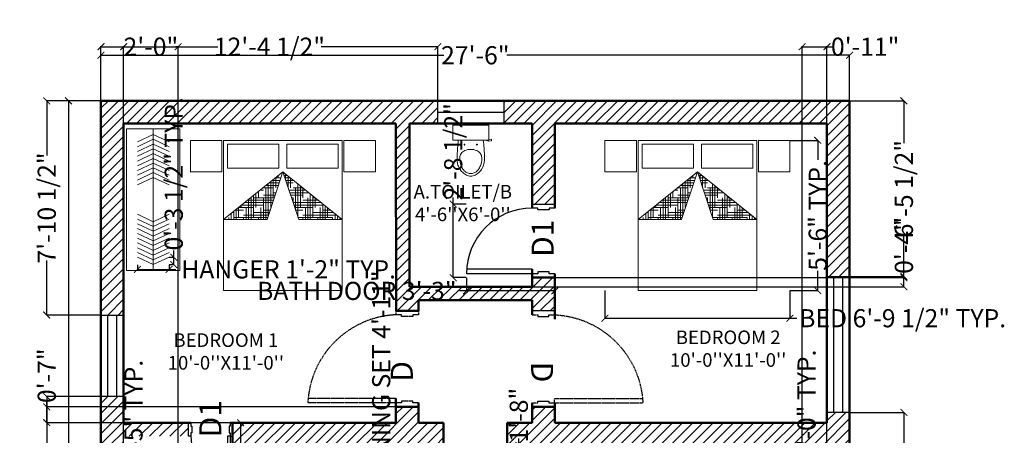
# Model space of a CAD drawing. Units: inches. Extents: x 1945 to 2401, y 1770 to 2289.
# Tile 5 of 5: x 1967 to 2401, y 2105 to 2289. Entities that reach past the tile are written whole.
import ezdxf

# ---------------------------------------------------------------- set-up
doc = ezdxf.new("R2010")
doc.units = ezdxf.units.IN
doc.linetypes.add('HIDDEN', pattern=[9.525, 6.35, -3.175])
for name, color, linetype, lineweight in [('A-ANNO-DIMS', 2, 'Continuous', 18), ('A-ANNO-TEXT', 7, 'Continuous', 18), ('A-AREA-IDEN', 7, 'Continuous', 25), ('A-DOOR-HIDN', 150, 'HIDDEN', 25), ('A-FLOR-FIXT', 9, 'Continuous', 18), ('A-WALL-PATT', 8, 'Continuous', 13), ('B-FURNITURE', 22, 'Continuous', 18), ('Doors', 150, 'Continuous', 25), ('shelves', 52, 'Continuous', 18), ('Walls', 7, 'Continuous', 50), ('Windows', 32, 'Continuous', 25)]:
    doc.layers.add(name, color=color, linetype=linetype, lineweight=lineweight)
doc.styles.get("Standard").update_dxf_attribs({"font": 'arial.ttf'})
doc.dimstyles.get("Standard").update_dxf_attribs({"dimtxt": 8, "dimasz": 3, "dimexe": 0.18, "dimexo": 0.0625, "dimgap": 0.09, "dimtad": 0, "dimdec": 1, "dimzin": 0, "dimdsep": 46, "dimlunit": 4, "dimtxsty": 'Standard', "dimblk": 'ARCHTICK', "dimcen": 0.09, "dimadec": 0, "dimazin": 0, "dimtfac": 1, "dimtdec": 1, "dimtofl": 0, "dimtmove": 0, "dimatfit": 3, "dimfxl": 1, "dimtolj": 1, "dimtzin": 0, "dimarcsym": 0})

# ---------------------------------------------------------------- blocks, each defined once
blk = doc.blocks.new('toilet-1')
at = {"color": 0, "linetype": 'ByBlock'}
for p, q in [((-0.23, -0.02), (-0.23, -0.212)), ((0.23, -0.02), (-0.23, -0.02)), ((0.23, -0.02), (0.23, -0.212)), ((-0.23, -0.212), (0.23, -0.212)), ((0.192, -0.214), (0.221, -0.225)), ((0.221, -0.225), (0.266, -0.219)), ((0.263, -0.2), (0.23, -0.204)), ((0.266, -0.219), (0.263, -0.2)), ((-0.089, -0.268), (-0.07, -0.268)), ((-0.079, -0.259), (-0.079, -0.278)), ((0.089, -0.268), (0.07, -0.268)), ((0.079, -0.259), (0.079, -0.278)), ((0, -0.638), (0, -0.638))]:
    blk.add_line(p, q, dxfattribs=at)
for centre, radius, start, end in [((3.527, -0.624), 3.709, 173.6925, 175.1593), ((-3.527, -0.624), 3.709, 4.8413, 6.3171), ((1.737, -0.452), 1.911, 175.7698, 180.3758), ((-0.031, -0.446), 0.111, 113.8997, 145.1485), ((0, -0.517), 0.188, 66.0939, 113.9061), ((0.031, -0.446), 0.111, 34.8515, 66.1003), ((-1.737, -0.452), 1.911, 359.6242, 4.2302), ((0.035, -0.463), 0.209, 180.3747, 194.3375), ((0.098, -0.45), 0.239, 175.8862, 195.5931), ((-0.041, -0.44), 0.0996, 145.1497, 175.881), ((0.041, -0.44), 0.0996, 4.119, 34.8503), ((-0.098, -0.45), 0.239, 344.4069, 4.1138), ((-0.035, -0.463), 0.209, 345.6614, 359.6243), ((0.055, -0.458), 0.23, 194.3353, 209.622), ((0.065, -0.452), 0.241, 209.6273, 224.5489), ((0.096, -0.45), 0.237, 195.5969, 209.3771), ((0.023, -0.491), 0.153, 209.3871, 226.5438), ((0.018, -0.499), 0.175, 224.552, 245.714), ((0.015, -0.5), 0.142, 226.5501, 246.5527), ((-0.015, -0.5), 0.142, 293.4473, 313.4499), ((-0.018, -0.499), 0.175, 294.2865, 315.4485), ((-0.023, -0.491), 0.153, 313.4562, 330.6129), ((-0.065, -0.452), 0.241, 315.4504, 330.372), ((-0.096, -0.45), 0.237, 330.6229, 344.4031), ((-0.055, -0.458), 0.23, 330.3788, 345.6655), ((0, -0.538), 0.132, 245.5845, 269.8782), ((0, -0.535), 0.103, 246.5493, 270.0042), ((0, -0.535), 0.103, 269.9958, 293.4507), ((0, -0.538), 0.132, 270.1216, 294.4153)]:
    blk.add_arc(centre, radius, start, end, dxfattribs=at)
blk = doc.blocks.new('AP0B05')
for p, q in [((35, 100), (35, 880)), ((75, 100), (75, 878.9))]:
    blk.add_line(p, q)
for points in [[(0, 100), (0, -100), (35, -100), (35, -50), (50, -50), (50, 50), (35, 50), (35, 100)], [(850, 100), (850, -100), (815, -100), (815, -50), (800, -50), (800, 50), (815, 50), (815, 100)]]:
    blk.add_lwpolyline(points, close=True)
blk.add_lwpolyline([(35, 100), (75, 100)])
blk.add_arc((-2.4, 62.6), 818.3, 2.62122, 87.37878)
blk = doc.blocks.new('AP0B01')
blk.add_line((75, 100), (75, 678.7))
blk.add_lwpolyline([(35, 100), (35, 680, -0.449922)], format="xyb")
for points in [[(0, 100), (0, -100), (35, -100), (35, -50), (50, -50), (50, 50), (35, 50), (35, 100)], [(650, 100), (650, -100), (615, -100), (615, -50), (600, -50), (600, 50), (615, 50), (615, 100)]]:
    blk.add_lwpolyline(points, close=True)
blk.add_lwpolyline([(35, 100), (75, 100)])
blk.add_arc((35, 100), 580, 0, 90)
blk = doc.blocks.new('*X11')
at = {"color": 0}
for p, q in [((20.125, 14.5), (20.125, 14.689)), ((20.149, 14.719), (20.277, 14.719)), ((20.156, 14.625), (20.156, 14.728)), ((20.174, 14.75), (20.277, 14.75)), ((20.188, 14.75), (20.188, 14.767)), ((20.199, 14.781), (20.277, 14.781)), ((20.25, 14.812), (20.277, 14.812)), ((20.25, 14.319), (20.25, 14.75)), ((20.031, 14.247), (20.031, 14.573)), ((20.062, 14.257), (20.062, 14.612)), ((20.094, 14.375), (20.094, 14.65)), ((20.098, 14.656), (20.125, 14.656)), ((20.124, 14.688), (20.25, 14.688)), ((20.125, 14.594), (20.277, 14.594)), ((20.219, 14.309), (20.219, 14.625)), ((20.25, 14.625), (20.277, 14.625)), ((19.948, 14.469), (20.125, 14.469)), ((19.973, 14.5), (20.25, 14.5)), ((19.998, 14.531), (20.277, 14.531)), ((20, 14.237), (20, 14.5)), ((20.023, 14.562), (20.277, 14.562)), ((20.188, 14.299), (20.188, 14.5)), ((19.844, 14.185), (19.844, 14.34)), ((19.875, 14.25), (19.875, 14.379)), ((19.875, 14.344), (20.277, 14.344)), ((19.906, 14.375), (19.906, 14.417)), ((19.922, 14.438), (20, 14.438)), ((19.969, 14.226), (19.969, 14.375)), ((20, 14.375), (20.277, 14.375)), ((20.125, 14.406), (20.277, 14.406)), ((20.156, 14.288), (20.156, 14.375)), ((20.25, 14.438), (20.277, 14.438)), ((19.746, 14.219), (19.875, 14.219)), ((19.75, 14.154), (19.75, 14.223)), ((19.772, 14.25), (20, 14.25)), ((19.781, 14.164), (19.781, 14.262)), ((19.797, 14.281), (20.125, 14.281)), ((19.812, 14.174), (19.812, 14.301)), ((19.822, 14.312), (20.229, 14.312)), ((19.938, 14.216), (19.938, 14.25)), ((19.702, 14.094), (19.779, 14.094)), ((19.719, 14.073), (19.719, 14.114)), ((19.721, 14.188), (19.75, 14.188)), ((19.75, 14.034), (19.75, 14.103)), ((19.781, 13.995), (19.781, 14.093)), ((19.812, 14), (19.812, 14.082)), ((19.727, 14.062), (19.873, 14.062)), ((19.752, 14.031), (19.875, 14.031)), ((19.875, 13.878), (19.875, 14)), ((19.875, 13.969), (20.156, 13.969)), ((19.906, 13.84), (19.906, 14.051)), ((19.938, 13.801), (19.938, 14.041)), ((19.969, 13.875), (19.969, 14.031)), ((20, 14), (20, 14.02)), ((20, 14), (20.061, 14)), ((20.062, 13.645), (20.062, 14)), ((20.094, 13.625), (20.094, 13.989)), ((20.125, 13.75), (20.125, 13.979)), ((20.156, 13.875), (20.156, 13.969)), ((19.827, 13.938), (20.25, 13.938)), ((19.853, 13.906), (20.125, 13.906)), ((19.878, 13.875), (20, 13.875)), ((20.031, 13.684), (20.031, 13.875)), ((20.125, 13.844), (20.277, 13.844)), ((20.219, 13.451), (20.219, 13.875)), ((20.25, 13.5), (20.25, 13.937)), ((20.25, 13.875), (20.277, 13.875)), ((19.953, 13.781), (20.277, 13.781)), ((19.978, 13.75), (20.25, 13.75)), ((20, 13.812), (20.277, 13.812)), ((20, 13.723), (20, 13.75)), ((20.003, 13.719), (20.125, 13.719)), ((20.188, 13.49), (20.188, 13.75)), ((20.079, 13.625), (20.277, 13.625)), ((20.104, 13.594), (20.277, 13.594)), ((20.125, 13.656), (20.277, 13.656)), ((20.156, 13.529), (20.156, 13.625)), ((20.25, 13.688), (20.277, 13.688)), ((20.129, 13.562), (20.25, 13.562)), ((20.205, 13.469), (20.277, 13.469)), ((20.25, 13.5), (20.277, 13.5)), ((20.23, 13.438), (20.277, 13.438)), ((20.255, 13.406), (20.277, 13.406))]:
    blk.add_line(p, q, dxfattribs=at)
blk = doc.blocks.new('MAT-P13')
for p, q in [((-1.17, 0), (-1.17, -0.4)), ((-1.17, 0), (-0.77, 0)), ((-0.77, 0), (-0.77, -0.4)), ((-0.75, 0), (0.75, 0)), ((-0.75, 0), (-0.75, -1.9)), ((0.75, 0), (0.75, -1.9)), ((0.77, 0), (1.17, 0)), ((0.77, 0), (0.77, -0.4)), ((1.17, 0), (1.17, -0.4)), ((-0.7, -0.05), (-0.7, -0.35)), ((-0.7, -0.05), (-0.05, -0.05)), ((-0.05, -0.35), (-0.05, -0.05)), ((0.05, -0.05), (0.7, -0.05)), ((0.05, -0.35), (0.05, -0.05)), ((0.7, -0.05), (0.7, -0.35)), ((-0.7, -0.35), (-0.05, -0.35)), ((0.05, -0.35), (0.7, -0.35)), ((-1.17, -0.4), (-0.77, -0.4)), ((-0.75, -1.003), (0, -0.4)), ((0, -0.4), (-0.75, -1.003)), ((0, -0.4), (-0.2, -1.003)), ((0, -0.4), (0.2, -1.003)), ((0, -0.4), (0.75, -1.003)), ((0.77, -0.4), (1.17, -0.4)), ((-0.75, -1.003), (-0.2, -1.003)), ((0.2, -1.003), (0.75, -1.003)), ((0.75, -1.9), (-0.75, -1.9))]:
    blk.add_line(p, q)
at = {"xscale": -1, "rotation": 90}
blk.add_blockref('*X11', (14.128, 19.274), dxfattribs=at)
blk = doc.blocks.new('_ArchTick')
at = {"color": 0, "linetype": 'ByBlock', "const_width": 0.15}
blk.add_lwpolyline([(-0.5, -0.5), (0.5, 0.5)], dxfattribs=at)
blk = doc.blocks.new('*D19')
at = {"layer": 'A-ANNO-DIMS', "color": 0, "lineweight": -2, "transparency": 16777216}
for p, q in [((2002.84, 2253.1), (2002.84, 2273.35)), ((2002.84, 2273.17), (2153.94, 2273.17)), ((2332.84, 2273.17), (2181.74, 2273.17)), ((2332.84, 2253.1), (2332.84, 2273.35))]:
    blk.add_line(p, q, dxfattribs=at)
at = {"layer": 'Defpoints', "color": 0, "transparency": 16777216}
for p in [(2332.84, 2273.17), (2002.84, 2253.04), (2332.84, 2253.04)]:
    blk.add_point(p, dxfattribs=at)
at = {"layer": 'A-ANNO-DIMS', "color": 0, "lineweight": -2, "transparency": 16777216, "xscale": 3, "yscale": 3, "zscale": 3, "rotation": 180}
blk.add_blockref('_ArchTick', (2002.84, 2273.17), dxfattribs=at)
at = {"layer": 'A-ANNO-DIMS', "color": 0, "lineweight": -2, "transparency": 16777216, "xscale": 3, "yscale": 3, "zscale": 3}
blk.add_blockref('_ArchTick', (2332.84, 2273.17), dxfattribs=at)
at = {"layer": 'A-ANNO-DIMS', "color": 0, "transparency": 16777216, "insert": (2167.84, 2273.17), "char_height": 8, "attachment_point": 5}
blk.add_mtext('\\A1;27\'-6"', dxfattribs=at)
blk = doc.blocks.new('*D20')
at = {"layer": 'A-ANNO-DIMS', "color": 0, "lineweight": -2, "transparency": 16777216}
for p, q in [((2002.78, 2253.04), (1988.38, 2253.04)), ((1988.56, 2253.04), (1988.56, 2043.37)), ((1988.56, 1806.04), (1988.56, 2015.71)), ((2002.78, 1806.04), (1988.38, 1806.04))]:
    blk.add_line(p, q, dxfattribs=at)
at = {"layer": 'Defpoints', "color": 0, "transparency": 16777216}
for p in [(2002.84, 2253.04), (1988.56, 1806.04), (2002.84, 1806.04)]:
    blk.add_point(p, dxfattribs=at)
at = {"layer": 'A-ANNO-DIMS', "color": 0, "lineweight": -2, "transparency": 16777216, "xscale": 3, "yscale": 3, "zscale": 3}
for p, rotation in [((1988.56, 2253.04), 90), ((1988.56, 1806.04), 270)]:
    blk.add_blockref('_ArchTick', p, dxfattribs=dict(at, rotation=rotation))
at = {"layer": 'A-ANNO-DIMS', "color": 0, "transparency": 16777216, "insert": (1988.56, 2029.54), "char_height": 8, "attachment_point": 5, "rotation": 90}
blk.add_mtext('\\A1;37\'-3"', dxfattribs=at)
blk = doc.blocks.new('WIN-60IN')
for p, q in [((0, 7), (60, 7)), ((0, 3), (60, 3))]:
    blk.add_line(p, q)
blk.add_lwpolyline([(0, 10), (60, 10), (60, 0), (0, 0)], close=True)
blk = doc.blocks.new('WIN-36IN')
for p, q in [((3, 0), (3, 36)), ((7, 0), (7, 36))]:
    blk.add_line(p, q)
blk.add_lwpolyline([(0, 0), (0, 36), (10, 36), (10, 0)], close=True)
blk = doc.blocks.new('VENT-WIN-29IN')
blk.add_line((0, 5), (29, 5))
blk.add_lwpolyline([(0, 10), (29, 10), (29, 0), (0, 0)], close=True)
blk = doc.blocks.new('WARDROBE-HANGER')
for q in [(0, 3.29), (13.91, 3.29)]:
    blk.add_line((6.95, 0), q)
blk = doc.blocks.new('*D27')
at = {"layer": 'A-ANNO-DIMS', "color": 0, "lineweight": -2, "transparency": 16777216}
for p, q in [((2018.93, 2180.72), (2018.93, 2178.52)), ((2018.93, 2178.7), (2032.84, 2178.7)), ((2032.84, 2180.72), (2032.84, 2178.52)), ((2032.84, 2178.7), (2035.84, 2178.7))]:
    blk.add_line(p, q, dxfattribs=at)
at = {"layer": 'Defpoints', "color": 0, "transparency": 16777216}
for p in [(2018.93, 2180.78), (2032.84, 2180.78), (2032.84, 2178.7)]:
    blk.add_point(p, dxfattribs=at)
at = {"layer": 'A-ANNO-DIMS', "color": 0, "lineweight": -2, "transparency": 16777216, "xscale": 3, "yscale": 3, "zscale": 3, "rotation": 180}
blk.add_blockref('_ArchTick', (2018.93, 2178.7), dxfattribs=at)
at = {"layer": 'A-ANNO-DIMS', "color": 0, "lineweight": -2, "transparency": 16777216, "xscale": 3, "yscale": 3, "zscale": 3}
blk.add_blockref('_ArchTick', (2032.84, 2178.7), dxfattribs=at)
at = {"layer": 'A-ANNO-DIMS', "color": 0, "transparency": 16777216, "insert": (2085.55, 2178.7), "char_height": 8, "attachment_point": 5}
blk.add_mtext('\\A1;HANGER 1\'-2" TYP.', dxfattribs=at)
blk = doc.blocks.new('*D28')
at = {"layer": 'A-ANNO-DIMS', "color": 0, "lineweight": -2, "transparency": 16777216}
for p, q in [((2032.9, 2184.07), (2035.1, 2184.07)), ((2034.92, 2184.07), (2034.92, 2187.07)), ((2034.92, 2180.78), (2034.92, 2184.07)), ((2032.9, 2180.78), (2035.1, 2180.78))]:
    blk.add_line(p, q, dxfattribs=at)
at = {"layer": 'Defpoints', "color": 0, "transparency": 16777216}
for p in [(2032.84, 2184.07), (2034.92, 2184.07), (2032.84, 2180.78)]:
    blk.add_point(p, dxfattribs=at)
at = {"layer": 'A-ANNO-DIMS', "color": 0, "lineweight": -2, "transparency": 16777216, "xscale": 3, "yscale": 3, "zscale": 3}
for p, rotation in [((2034.92, 2184.07), 90), ((2034.92, 2180.78), 270)]:
    blk.add_blockref('_ArchTick', p, dxfattribs=dict(at, rotation=rotation))
at = {"layer": 'A-ANNO-DIMS', "color": 0, "transparency": 16777216, "insert": (2034.92, 2220.86), "char_height": 8, "attachment_point": 5, "rotation": 90}
blk.add_mtext('\\A1;0\'-3 1/2" TYP.', dxfattribs=at)
blk = doc.blocks.new('*D35')
at = {"layer": 'A-ANNO-DIMS', "color": 0, "lineweight": -2, "transparency": 16777216}
for p, q in [((2322.78, 2041.04), (2313.66, 2041.04)), ((2313.84, 2041.04), (2313.84, 2044.04)), ((2313.84, 1981.04), (2313.84, 2041.04)), ((2322.78, 1981.04), (2313.66, 1981.04))]:
    blk.add_line(p, q, dxfattribs=at)
at = {"layer": 'Defpoints', "color": 0, "transparency": 16777216}
for p in [(2313.84, 2041.04), (2322.84, 2041.04), (2322.84, 1981.04)]:
    blk.add_point(p, dxfattribs=at)
at = {"layer": 'A-ANNO-DIMS', "color": 0, "lineweight": -2, "transparency": 16777216, "xscale": 3, "yscale": 3, "zscale": 3}
for p, rotation in [((2313.84, 2041.04), 90), ((2313.84, 1981.04), 270)]:
    blk.add_blockref('_ArchTick', p, dxfattribs=dict(at, rotation=rotation))
at = {"layer": 'A-ANNO-DIMS', "color": 0, "transparency": 16777216, "insert": (2313.84, 2094.75), "char_height": 8, "attachment_point": 5, "rotation": 90}
blk.add_mtext('\\A1;WINDOW 5\'-0" TYP.', dxfattribs=at)
blk = doc.blocks.new('*D43')
at = {"layer": 'A-ANNO-DIMS', "color": 0, "lineweight": -2, "transparency": 16777216}
for p, q in [((2060.9, 2111.04), (2064.52, 2111.04)), ((2064.34, 2111.04), (2064.34, 2087.72)), ((2060.9, 2087.72), (2064.52, 2087.72)), ((2064.34, 2087.72), (2064.34, 2084.72))]:
    blk.add_line(p, q, dxfattribs=at)
at = {"layer": 'Defpoints', "color": 0, "transparency": 16777216}
for p in [(2060.84, 2111.04), (2060.84, 2087.72), (2064.34, 2087.72)]:
    blk.add_point(p, dxfattribs=at)
at = {"layer": 'A-ANNO-DIMS', "color": 0, "lineweight": -2, "transparency": 16777216, "xscale": 3, "yscale": 3, "zscale": 3}
for p, rotation in [((2064.34, 2111.04), 90), ((2064.34, 2087.72), 270)]:
    blk.add_blockref('_ArchTick', p, dxfattribs=dict(at, rotation=rotation))
at = {"layer": 'A-ANNO-DIMS', "color": 0, "transparency": 16777216, "insert": (2064.34, 2026.98), "char_height": 8, "attachment_point": 5, "rotation": 90}
blk.add_mtext('\\A1;BATH DOOR 1\'-11 1/2"', dxfattribs=at)
blk = doc.blocks.new('*D45')
at = {"layer": 'A-ANNO-DIMS', "color": 0, "lineweight": -2, "transparency": 16777216}
for p, q in [((2163.93, 2174.98), (2163.93, 2169.02)), ((2202.84, 2174.98), (2202.84, 2169.02)), ((2163.93, 2169.2), (2160.93, 2169.2)), ((2202.84, 2169.2), (2163.93, 2169.2))]:
    blk.add_line(p, q, dxfattribs=at)
at = {"layer": 'Defpoints', "color": 0, "transparency": 16777216}
for p in [(2163.93, 2175.04), (2202.84, 2175.04), (2163.93, 2169.2)]:
    blk.add_point(p, dxfattribs=at)
at = {"layer": 'A-ANNO-DIMS', "color": 0, "lineweight": -2, "transparency": 16777216, "xscale": 3, "yscale": 3, "zscale": 3, "rotation": 180}
blk.add_blockref('_ArchTick', (2163.93, 2169.2), dxfattribs=at)
at = {"layer": 'A-ANNO-DIMS', "color": 0, "lineweight": -2, "transparency": 16777216, "xscale": 3, "yscale": 3, "zscale": 3}
blk.add_blockref('_ArchTick', (2202.84, 2169.2), dxfattribs=at)
at = {"layer": 'A-ANNO-DIMS', "color": 0, "transparency": 16777216, "insert": (2115.61, 2169.2), "char_height": 8, "attachment_point": 5}
blk.add_mtext('\\A1;BATH DOOR 3\'-3"', dxfattribs=at)
blk = doc.blocks.new('*D46')
at = {"layer": 'A-ANNO-DIMS', "color": 0, "lineweight": -2, "transparency": 16777216}
for p, q in [((2158.1, 2207.47), (2158.1, 2210.47)), ((2163.87, 2207.47), (2157.92, 2207.47)), ((2158.1, 2175.04), (2158.1, 2207.47)), ((2163.87, 2175.04), (2157.92, 2175.04))]:
    blk.add_line(p, q, dxfattribs=at)
at = {"layer": 'Defpoints', "color": 0, "transparency": 16777216}
for p in [(2158.1, 2207.47), (2163.93, 2207.47), (2163.93, 2175.04)]:
    blk.add_point(p, dxfattribs=at)
at = {"layer": 'A-ANNO-DIMS', "color": 0, "lineweight": -2, "transparency": 16777216, "xscale": 3, "yscale": 3, "zscale": 3}
for p, rotation in [((2158.1, 2207.47), 90), ((2158.1, 2175.04), 270)]:
    blk.add_blockref('_ArchTick', p, dxfattribs=dict(at, rotation=rotation))
at = {"layer": 'A-ANNO-DIMS', "color": 0, "transparency": 16777216, "insert": (2158.1, 2230.58), "char_height": 8, "attachment_point": 5, "rotation": 90}
blk.add_mtext('\\A1;2\'-8 1/2"', dxfattribs=at)
blk = doc.blocks.new('*D47')
at = {"layer": 'A-ANNO-DIMS', "color": 0, "lineweight": -2, "transparency": 16777216}
for p, q in [((2224.95, 2169.32), (2224.95, 2156.96)), ((2306.53, 2169.32), (2306.53, 2156.96)), ((2224.95, 2157.14), (2306.53, 2157.14)), ((2306.53, 2157.14), (2309.53, 2157.14))]:
    blk.add_line(p, q, dxfattribs=at)
at = {"layer": 'Defpoints', "color": 0, "transparency": 16777216}
for p in [(2224.95, 2169.38), (2306.53, 2169.38), (2306.53, 2157.14)]:
    blk.add_point(p, dxfattribs=at)
at = {"layer": 'A-ANNO-DIMS', "color": 0, "lineweight": -2, "transparency": 16777216, "xscale": 3, "yscale": 3, "zscale": 3, "rotation": 180}
blk.add_blockref('_ArchTick', (2224.95, 2157.14), dxfattribs=at)
at = {"layer": 'A-ANNO-DIMS', "color": 0, "lineweight": -2, "transparency": 16777216, "xscale": 3, "yscale": 3, "zscale": 3}
blk.add_blockref('_ArchTick', (2306.53, 2157.14), dxfattribs=at)
at = {"layer": 'A-ANNO-DIMS', "color": 0, "transparency": 16777216, "insert": (2356.19, 2157.14), "char_height": 8, "attachment_point": 5}
blk.add_mtext('\\A1;BED 6\'-9 1/2" TYP.', dxfattribs=at)
blk = doc.blocks.new('*D48')
at = {"layer": 'A-ANNO-DIMS', "color": 0, "lineweight": -2, "transparency": 16777216}
for p, q in [((2306.59, 2235.62), (2318.95, 2235.62)), ((2318.77, 2235.62), (2318.77, 2226.97)), ((2318.77, 2169.38), (2318.77, 2178.03)), ((2306.59, 2169.38), (2318.95, 2169.38))]:
    blk.add_line(p, q, dxfattribs=at)
at = {"layer": 'Defpoints', "color": 0, "transparency": 16777216}
for p in [(2306.53, 2235.62), (2318.77, 2235.62), (2306.53, 2169.38)]:
    blk.add_point(p, dxfattribs=at)
at = {"layer": 'A-ANNO-DIMS', "color": 0, "lineweight": -2, "transparency": 16777216, "xscale": 3, "yscale": 3, "zscale": 3}
for p, rotation in [((2318.77, 2235.62), 90), ((2318.77, 2169.38), 270)]:
    blk.add_blockref('_ArchTick', p, dxfattribs=dict(at, rotation=rotation))
at = {"layer": 'A-ANNO-DIMS', "color": 0, "transparency": 16777216, "insert": (2318.77, 2202.5), "char_height": 8, "attachment_point": 5, "rotation": 90}
blk.add_mtext('\\A1;5\'-6" TYP.', dxfattribs=at)
blk = doc.blocks.new('*D51')
at = {"layer": 'A-ANNO-DIMS', "color": 0, "lineweight": -2, "transparency": 16777216}
for p, q in [((2017.19, 2055.45), (2017.19, 2058.45)), ((2012.9, 2055.45), (2017.37, 2055.45)), ((2017.19, 2026.45), (2017.19, 2055.45)), ((2012.9, 2026.45), (2017.37, 2026.45))]:
    blk.add_line(p, q, dxfattribs=at)
at = {"layer": 'Defpoints', "color": 0, "transparency": 16777216}
for p in [(2012.84, 2055.45), (2017.19, 2055.45), (2012.84, 2026.45)]:
    blk.add_point(p, dxfattribs=at)
at = {"layer": 'A-ANNO-DIMS', "color": 0, "lineweight": -2, "transparency": 16777216, "xscale": 3, "yscale": 3, "zscale": 3}
for p, rotation in [((2017.19, 2055.45), 90), ((2017.19, 2026.45), 270)]:
    blk.add_blockref('_ArchTick', p, dxfattribs=dict(at, rotation=rotation))
at = {"layer": 'A-ANNO-DIMS', "color": 0, "transparency": 16777216, "insert": (2017.19, 2099.59), "char_height": 8, "attachment_point": 5, "rotation": 90}
blk.add_mtext('\\A1;VENT 2\'-5" TYP.', dxfattribs=at)
blk = doc.blocks.new('*D53')
at = {"layer": 'A-ANNO-DIMS', "color": 0, "lineweight": -2, "transparency": 16777216}
for p, q in [((2126.35, 2082.22), (2126.35, 2085.22)), ((2117.54, 2082.22), (2126.53, 2082.22)), ((2126.35, 2023.05), (2126.35, 2082.22)), ((2117.54, 2023.05), (2126.53, 2023.05))]:
    blk.add_line(p, q, dxfattribs=at)
at = {"layer": 'Defpoints', "color": 0, "transparency": 16777216}
for p in [(2117.47, 2082.22), (2126.35, 2082.22), (2117.47, 2023.05)]:
    blk.add_point(p, dxfattribs=at)
at = {"layer": 'A-ANNO-DIMS', "color": 0, "lineweight": -2, "transparency": 16777216, "xscale": 3, "yscale": 3, "zscale": 3}
for p, rotation in [((2126.35, 2082.22), 90), ((2126.35, 2023.05), 270)]:
    blk.add_blockref('_ArchTick', p, dxfattribs=dict(at, rotation=rotation))
at = {"layer": 'A-ANNO-DIMS', "color": 0, "transparency": 16777216, "insert": (2126.35, 2132.38), "char_height": 8, "attachment_point": 5, "rotation": 90}
blk.add_mtext('\\A1;DINING SET 4\'-11"', dxfattribs=at)
blk = doc.blocks.new('*D56')
at = {"layer": 'A-ANNO-DIMS', "color": 0, "lineweight": -2, "transparency": 16777216}
for p, q in [((2195.52, 2101.04), (2186.82, 2101.04)), ((2187, 2101.04), (2187, 2104.04)), ((2187, 2080.88), (2187, 2101.04)), ((2195.52, 2080.88), (2186.82, 2080.88))]:
    blk.add_line(p, q, dxfattribs=at)
at = {"layer": 'Defpoints', "color": 0, "transparency": 16777216}
for p in [(2187, 2101.04), (2195.59, 2101.04), (2195.59, 2080.88)]:
    blk.add_point(p, dxfattribs=at)
at = {"layer": 'A-ANNO-DIMS', "color": 0, "lineweight": -2, "transparency": 16777216, "xscale": 3, "yscale": 3, "zscale": 3}
for p, rotation in [((2187, 2101.04), 90), ((2187, 2080.88), 270)]:
    blk.add_blockref('_ArchTick', p, dxfattribs=dict(at, rotation=rotation))
at = {"layer": 'A-ANNO-DIMS', "color": 0, "transparency": 16777216, "insert": (2187, 2114.39), "char_height": 8, "attachment_point": 5, "rotation": 90}
blk.add_mtext('\\A1;1\'-8"', dxfattribs=at)
blk = doc.blocks.new('*D59')
at = {"layer": 'A-ANNO-DIMS', "color": 0, "lineweight": -2, "transparency": 16777216}
for p, q in [((2002.84, 2253.1), (2002.84, 2277.12)), ((2002.84, 2276.94), (2054.32, 2276.94)), ((2151.34, 2276.94), (2099.87, 2276.94)), ((2151.34, 2253.1), (2151.34, 2277.12))]:
    blk.add_line(p, q, dxfattribs=at)
at = {"layer": 'Defpoints', "color": 0, "transparency": 16777216}
for p in [(2151.34, 2276.94), (2002.84, 2253.04), (2151.34, 2253.04)]:
    blk.add_point(p, dxfattribs=at)
at = {"layer": 'A-ANNO-DIMS', "color": 0, "lineweight": -2, "transparency": 16777216, "xscale": 3, "yscale": 3, "zscale": 3, "rotation": 180}
blk.add_blockref('_ArchTick', (2002.84, 2276.94), dxfattribs=at)
at = {"layer": 'A-ANNO-DIMS', "color": 0, "lineweight": -2, "transparency": 16777216, "xscale": 3, "yscale": 3, "zscale": 3}
blk.add_blockref('_ArchTick', (2151.34, 2276.94), dxfattribs=at)
at = {"layer": 'A-ANNO-DIMS', "color": 0, "transparency": 16777216, "insert": (2077.09, 2276.94), "char_height": 8, "attachment_point": 5}
blk.add_mtext('\\A1;12\'-4 1/2"', dxfattribs=at)
blk = doc.blocks.new('*D60')
at = {"layer": 'A-ANNO-DIMS', "color": 0, "lineweight": -2, "transparency": 16777216}
for p, q in [((2332.9, 2253.04), (2356.92, 2253.04)), ((2356.74, 2253.04), (2356.74, 2234.37)), ((2356.74, 2175.57), (2356.74, 2194.24)), ((2332.9, 2175.57), (2356.92, 2175.57))]:
    blk.add_line(p, q, dxfattribs=at)
at = {"layer": 'Defpoints', "color": 0, "transparency": 16777216}
for p in [(2332.84, 2253.04), (2332.84, 2175.57), (2356.74, 2175.57)]:
    blk.add_point(p, dxfattribs=at)
at = {"layer": 'A-ANNO-DIMS', "color": 0, "lineweight": -2, "transparency": 16777216, "xscale": 3, "yscale": 3, "zscale": 3}
for p, rotation in [((2356.74, 2253.04), 90), ((2356.74, 2175.57), 270)]:
    blk.add_blockref('_ArchTick', p, dxfattribs=dict(at, rotation=rotation))
at = {"layer": 'A-ANNO-DIMS', "color": 0, "transparency": 16777216, "insert": (2356.74, 2214.3), "char_height": 8, "attachment_point": 5, "rotation": 90}
blk.add_mtext('\\A1;6\'-5 1/2"', dxfattribs=at)
blk = doc.blocks.new('*D61')
at = {"layer": 'A-ANNO-DIMS', "color": 0, "lineweight": -2, "transparency": 16777216}
for p, q in [((2332.9, 2115.57), (2356.92, 2115.57)), ((2356.74, 2115.57), (2356.74, 2098.37)), ((2356.74, 2041.04), (2356.74, 2058.24)), ((2332.9, 2041.04), (2356.92, 2041.04))]:
    blk.add_line(p, q, dxfattribs=at)
at = {"layer": 'Defpoints', "color": 0, "transparency": 16777216}
for p in [(2332.84, 2115.57), (2332.84, 2041.04), (2356.74, 2041.04)]:
    blk.add_point(p, dxfattribs=at)
at = {"layer": 'A-ANNO-DIMS', "color": 0, "lineweight": -2, "transparency": 16777216, "xscale": 3, "yscale": 3, "zscale": 3}
for p, rotation in [((2356.74, 2115.57), 90), ((2356.74, 2041.04), 270)]:
    blk.add_blockref('_ArchTick', p, dxfattribs=dict(at, rotation=rotation))
at = {"layer": 'A-ANNO-DIMS', "color": 0, "transparency": 16777216, "insert": (2356.74, 2078.3), "char_height": 8, "attachment_point": 5, "rotation": 90}
blk.add_mtext('\\A1;6\'-2 1/2"', dxfattribs=at)
blk = doc.blocks.new('*D62')
at = {"layer": 'A-ANNO-DIMS', "color": 0, "lineweight": -2, "transparency": 16777216}
for p, q in [((2002.78, 2253.04), (1978.76, 2253.04)), ((1978.94, 2253.04), (1978.94, 2228.91)), ((1978.94, 2158.54), (1978.94, 2182.67)), ((2002.78, 2158.54), (1978.76, 2158.54))]:
    blk.add_line(p, q, dxfattribs=at)
at = {"layer": 'Defpoints', "color": 0, "transparency": 16777216}
for p in [(2002.84, 2253.04), (1978.94, 2158.54), (2002.84, 2158.54)]:
    blk.add_point(p, dxfattribs=at)
at = {"layer": 'A-ANNO-DIMS', "color": 0, "lineweight": -2, "transparency": 16777216, "xscale": 3, "yscale": 3, "zscale": 3}
for p, rotation in [((1978.94, 2253.04), 90), ((1978.94, 2158.54), 270)]:
    blk.add_blockref('_ArchTick', p, dxfattribs=dict(at, rotation=rotation))
at = {"layer": 'A-ANNO-DIMS', "color": 0, "transparency": 16777216, "insert": (1978.94, 2205.79), "char_height": 8, "attachment_point": 5, "rotation": 90}
blk.add_mtext('\\A1;7\'-10 1/2"', dxfattribs=at)
blk = doc.blocks.new('*D63')
at = {"layer": 'A-ANNO-DIMS', "color": 0, "lineweight": -2, "transparency": 16777216}
for p, q in [((2002.78, 2122.54), (1978.76, 2122.54)), ((1978.94, 2122.54), (1978.94, 2099.72)), ((1978.94, 2055.45), (1978.94, 2078.27)), ((2002.78, 2055.45), (1978.76, 2055.45))]:
    blk.add_line(p, q, dxfattribs=at)
at = {"layer": 'Defpoints', "color": 0, "transparency": 16777216}
for p in [(2002.84, 2122.54), (1978.94, 2055.45), (2002.84, 2055.45)]:
    blk.add_point(p, dxfattribs=at)
at = {"layer": 'A-ANNO-DIMS', "color": 0, "lineweight": -2, "transparency": 16777216, "xscale": 3, "yscale": 3, "zscale": 3}
for p, rotation in [((1978.94, 2122.54), 90), ((1978.94, 2055.45), 270)]:
    blk.add_blockref('_ArchTick', p, dxfattribs=dict(at, rotation=rotation))
at = {"layer": 'A-ANNO-DIMS', "color": 0, "transparency": 16777216, "insert": (1978.94, 2089), "char_height": 8, "attachment_point": 5, "rotation": 90}
blk.add_mtext('\\A1;5\'-7"', dxfattribs=at)
blk = doc.blocks.new('*D66')
at = {"layer": 'A-ANNO-DIMS', "color": 0, "lineweight": -2, "transparency": 16777216}
for p, q in [((2311.84, 1921.1), (2311.84, 2277.12)), ((2311.84, 2276.94), (2322.84, 2276.94)), ((2322.84, 1921.1), (2322.84, 2277.12)), ((2322.84, 2276.94), (2325.84, 2276.94))]:
    blk.add_line(p, q, dxfattribs=at)
at = {"layer": 'Defpoints', "color": 0, "transparency": 16777216}
for p in [(2322.84, 2276.94), (2311.84, 1921.04), (2322.84, 1921.04)]:
    blk.add_point(p, dxfattribs=at)
at = {"layer": 'A-ANNO-DIMS', "color": 0, "lineweight": -2, "transparency": 16777216, "xscale": 3, "yscale": 3, "zscale": 3, "rotation": 180}
blk.add_blockref('_ArchTick', (2311.84, 2276.94), dxfattribs=at)
at = {"layer": 'A-ANNO-DIMS', "color": 0, "lineweight": -2, "transparency": 16777216, "xscale": 3, "yscale": 3, "zscale": 3}
blk.add_blockref('_ArchTick', (2322.84, 2276.94), dxfattribs=at)
at = {"layer": 'A-ANNO-DIMS', "color": 0, "transparency": 16777216, "insert": (2339.67, 2276.94), "char_height": 8, "attachment_point": 5}
blk.add_mtext('\\A1;0\'-11"', dxfattribs=at)
blk = doc.blocks.new('*D67')
at = {"layer": 'A-ANNO-DIMS', "color": 0, "lineweight": -2, "transparency": 16777216}
for p, q in [((2012.84, 1931.1), (2012.84, 2277.12)), ((2012.84, 2276.94), (2014.05, 2276.94)), ((2036.84, 2276.94), (2035.63, 2276.94)), ((2036.84, 1922.1), (2036.84, 2277.12))]:
    blk.add_line(p, q, dxfattribs=at)
at = {"layer": 'Defpoints', "color": 0, "transparency": 16777216}
for p in [(2036.84, 2276.94), (2012.84, 1931.04), (2036.84, 1922.04)]:
    blk.add_point(p, dxfattribs=at)
at = {"layer": 'A-ANNO-DIMS', "color": 0, "lineweight": -2, "transparency": 16777216, "xscale": 3, "yscale": 3, "zscale": 3, "rotation": 180}
blk.add_blockref('_ArchTick', (2012.84, 2276.94), dxfattribs=at)
at = {"layer": 'A-ANNO-DIMS', "color": 0, "lineweight": -2, "transparency": 16777216, "xscale": 3, "yscale": 3, "zscale": 3}
blk.add_blockref('_ArchTick', (2036.84, 2276.94), dxfattribs=at)
at = {"layer": 'A-ANNO-DIMS', "color": 0, "transparency": 16777216, "insert": (2024.84, 2276.94), "char_height": 8, "attachment_point": 5}
blk.add_mtext('\\A1;2\'-0"', dxfattribs=at)
blk = doc.blocks.new('*D71')
at = {"layer": 'A-ANNO-DIMS', "color": 0, "lineweight": -2, "transparency": 16777216}
for p, q in [((2132.78, 2118.04), (1978.76, 2118.04)), ((1978.94, 2118.04), (1978.94, 2121.04)), ((1978.94, 2111.04), (1978.94, 2118.04)), ((2132.78, 2111.04), (1978.76, 2111.04))]:
    blk.add_line(p, q, dxfattribs=at)
at = {"layer": 'Defpoints', "color": 0, "transparency": 16777216}
for p in [(1978.94, 2118.04), (2132.84, 2118.04), (2132.84, 2111.04)]:
    blk.add_point(p, dxfattribs=at)
at = {"layer": 'A-ANNO-DIMS', "color": 0, "lineweight": -2, "transparency": 16777216, "xscale": 3, "yscale": 3, "zscale": 3}
for p, rotation in [((1978.94, 2118.04), 90), ((1978.94, 2111.04), 270)]:
    blk.add_blockref('_ArchTick', p, dxfattribs=dict(at, rotation=rotation))
at = {"layer": 'A-ANNO-DIMS', "color": 0, "transparency": 16777216, "insert": (1978.94, 2131.76), "char_height": 8, "attachment_point": 5, "rotation": 90}
blk.add_mtext('\\A1;0\'-7"', dxfattribs=at)
blk = doc.blocks.new('*D72')
at = {"layer": 'A-ANNO-DIMS', "color": 0, "lineweight": -2, "transparency": 16777216}
for p, q in [((2192.9, 2175.04), (2356.92, 2175.04)), ((2356.74, 2175.04), (2356.74, 2178.04)), ((2356.74, 2171.04), (2356.74, 2175.04)), ((2192.9, 2171.04), (2356.92, 2171.04))]:
    blk.add_line(p, q, dxfattribs=at)
at = {"layer": 'Defpoints', "color": 0, "transparency": 16777216}
for p in [(2192.84, 2175.04), (2356.74, 2175.04), (2192.84, 2171.04)]:
    blk.add_point(p, dxfattribs=at)
at = {"layer": 'A-ANNO-DIMS', "color": 0, "lineweight": -2, "transparency": 16777216, "xscale": 3, "yscale": 3, "zscale": 3}
for p, rotation in [((2356.74, 2175.04), 90), ((2356.74, 2171.04), 270)]:
    blk.add_blockref('_ArchTick', p, dxfattribs=dict(at, rotation=rotation))
at = {"layer": 'A-ANNO-DIMS', "color": 0, "transparency": 16777216, "insert": (2356.74, 2188.76), "char_height": 8, "attachment_point": 5, "rotation": 90}
blk.add_mtext('\\A1;0\'-4"', dxfattribs=at)

msp = doc.modelspace()

# ---------------------------------------------------------------- hatches: boundary and pattern name
at = {"layer": 'A-WALL-PATT', "transparency": 33554585}
h = msp.add_hatch(dxfattribs=at)
h.set_pattern_fill('ANSI31', color=256)
h.paths.add_polyline_path([(2151.34, 2253.04), (2002.84, 2253.04), (2002.84, 2158.54), (2012.84, 2158.54), (2012.84, 2243.04), (2132.84, 2243.04), (2132.88, 2160.39), (2142.84, 2160.39), (2142.84, 2165.04), (2192.84, 2165.04), (2192.84, 2160.39), (2202.84, 2160.39), (2202.84, 2175.04), (2192.84, 2175.04), (2192.84, 2171.04), (2138.84, 2171.04), (2138.84, 2243.04), (2151.34, 2243.04)])
h.paths.add_polyline_path([(2332.84, 2253.04), (2180.34, 2253.04), (2180.34, 2243.04), (2192.84, 2243.04), (2192.84, 2207.47), (2202.84, 2207.47), (2202.84, 2243.04), (2322.84, 2243.04), (2322.84, 2175.57), (2332.84, 2175.57)])
h.paths.add_polyline_path([(2012.84, 2105.04), (2041.41, 2105.04), (2041.41, 2111.04), (2012.84, 2111.04), (2012.84, 2122.54), (2002.84, 2122.54), (2002.84, 2055.45), (2012.84, 2055.45)])
h.paths.add_polyline_path([(2332.84, 2115.57), (2322.84, 2115.57), (2322.84, 2111.04), (2202.84, 2111.04), (2202.84, 2118.04), (2192.84, 2118.04), (2192.84, 2111.04), (2181.84, 2111.04), (2181.84, 2101.04), (2322.84, 2101.04), (2322.84, 2041.04), (2332.84, 2041.04)])
h = msp.add_hatch(dxfattribs=at)
h.set_pattern_fill('ANSI31', color=256)
h.paths.add_polyline_path([(2142.84, 2006.04), (2132.84, 2006.04), (2132.84, 1898.04), (2012.84, 1898.04), (2012.84, 1888.04), (2142.84, 1888.04), (2142.84, 1911.04), (2179.42, 1911.04), (2179.42, 1921.04), (2142.84, 1921.04)])
h.paths.add_polyline_path([(2269.5, 1921.04), (2239.42, 1921.04), (2239.42, 1911.04), (2269.5, 1911.04)])
h.paths.add_polyline_path([(2332.84, 1981.04), (2322.84, 1981.04), (2322.84, 1921.04), (2311.84, 1921.04), (2311.84, 1911.04), (2322.84, 1911.04), (2322.84, 1817.97), (2332.84, 1817.97)])
h.paths.add_polyline_path([(2012.84, 1931.04), (2002.84, 1931.04), (2002.84, 1806.04), (2142.84, 1806.04), (2142.84, 1816.04), (2012.84, 1816.04)])
h.paths.add_polyline_path([(2012.84, 2000.04), (2082.92, 2000.04), (2082.92, 2006.04), (2066.84, 2006.04), (2066.84, 2101.04), (2142.84, 2101.04), (2153.84, 2101.04), (2153.84, 2111.04), (2142.84, 2111.04), (2142.84, 2118.04), (2132.84, 2118.04), (2132.84, 2111.04), (2060.84, 2111.04), (2060.84, 2006.04), (2012.84, 2006.04), (2012.84, 2026.45), (2002.84, 2026.45), (2002.84, 1967.04), (2012.84, 1967.04)])

# ---------------------------------------------------------------- linework, layer by layer
at = {"layer": 'shelves'}
msp.add_line((2025.88, 2240.72), (2025.88, 2178.25), dxfattribs=at)
msp.add_lwpolyline([(2014.15, 2240.72), (2037.62, 2240.72), (2037.62, 2178.25), (2014.15, 2178.25)], close=True, dxfattribs=at)
at = {"layer": 'Walls'}
for p, q in [((2002.84, 2253.04), (2332.84, 2253.04)), ((2002.84, 2253.04), (2002.84, 1806.04)), ((2332.84, 2253.04), (2332.84, 1805.97)), ((2012.84, 2243.04), (2132.84, 2243.04)), ((2012.84, 2243.04), (2012.84, 2111.04)), ((2132.84, 2243.04), (2132.88, 2160.39)), ((2138.84, 2243.04), (2138.84, 2171.04)), ((2138.84, 2243.04), (2192.84, 2243.04)), ((2192.84, 2243.04), (2192.84, 2205.72)), ((2202.84, 2243.04), (2202.84, 2205.72)), ((2202.84, 2243.04), (2322.84, 2243.04)), ((2322.84, 2243.04), (2322.84, 2111.04)), ((2192.84, 2178.78), (2192.84, 2171.04)), ((2192.84, 2175.04), (2202.84, 2175.04)), ((2202.84, 2176.79), (2202.84, 2156.65)), ((2138.84, 2171.04), (2192.84, 2171.04)), ((2142.84, 2165.04), (2192.84, 2165.04)), ((2142.84, 2160.39), (2142.84, 2165.04)), ((2192.84, 2165.04), (2192.84, 2158.64)), ((2132.88, 2160.39), (2142.84, 2160.39)), ((2132.84, 2121.78), (2132.84, 2111.04)), ((2132.84, 2118.04), (2142.84, 2118.04)), ((2142.84, 2119.78), (2142.84, 2111.04)), ((2192.84, 2119.78), (2192.84, 2111.04)), ((2192.84, 2118.04), (2202.84, 2118.04)), ((2202.84, 2119.79), (2202.84, 2111.04)), ((2012.84, 2111.04), (2042.46, 2111.04)), ((2059.8, 2111.04), (2132.84, 2111.04)), ((2060.84, 2111.04), (2060.84, 2006.04)), ((2142.84, 2111.04), (2153.84, 2111.04)), ((2153.84, 2111.04), (2153.84, 2101.04)), ((2192.84, 2111.04), (2181.84, 2111.04)), ((2181.84, 2111.04), (2181.84, 2101.04)), ((2202.84, 2111.04), (2322.84, 2111.04))]:
    msp.add_line(p, q, dxfattribs=at)

# ---------------------------------------------------------------- block references
at = {"layer": 'A-DOOR-HIDN', "yscale": 0.0498193668704145, "zscale": 0.0498193668704145}
for p, xscale, rotation in [((2137.86, 2118.04), 0.0498193668704145, 90.00000000000003), ((2197.82, 2118.04), -0.0498193668704145, 270)]:
    msp.add_blockref('AP0B05', p, dxfattribs=dict(at, xscale=xscale, rotation=rotation))
at = {"layer": 'A-FLOR-FIXT', "xscale": 34.59924330403631, "yscale": 34.59924330403631, "zscale": 34.59924330403631}
msp.add_blockref('toilet-1', (2165.84, 2243.04), dxfattribs=at)
at = {"layer": 'B-FURNITURE', "xscale": 34.86441752320295, "yscale": 34.86441752320295, "zscale": 34.86441752320295}
for p in [(2083.02, 2235.62), (2265.74, 2235.62)]:
    msp.add_blockref('MAT-P13', p, dxfattribs=at)
at = {"layer": 'Doors'}
for p, xscale, yscale, zscale, rotation in [((2197.85, 2175.04), 0.0498850584424388, 0.0498850584424388, 0.0498850584424388, 90), ((2060.84, 2108.05), 0.0298912553794466, 0.0298912553794466, 0.0298912553794466, 180)]:
    msp.add_blockref('AP0B01', p, dxfattribs=dict(at, xscale=xscale, yscale=yscale, zscale=zscale, rotation=rotation))
at = {"layer": 'shelves', "rotation": 180}
for p in [(2032.84, 2238.19), (2032.84, 2236.09), (2032.84, 2233.99), (2032.84, 2231.88), (2032.84, 2229.78), (2032.84, 2227.68), (2032.84, 2225.58), (2032.84, 2223.48), (2032.84, 2221.38), (2032.84, 2219.28)]:
    msp.add_blockref('WARDROBE-HANGER', p, dxfattribs=at)
at = {"layer": 'shelves'}
for p in [(2018.93, 2199.69), (2018.93, 2197.59), (2018.93, 2195.49), (2018.93, 2193.39), (2018.93, 2191.29), (2018.93, 2189.19), (2018.93, 2187.09), (2018.93, 2184.98), (2018.93, 2182.88), (2018.93, 2180.78)]:
    msp.add_blockref('WARDROBE-HANGER', p, dxfattribs=at)
at = {"layer": 'Windows'}
for name, p in [('VENT-WIN-29IN', (2151.34, 2243.04)), ('WIN-36IN', (2002.84, 2122.54))]:
    msp.add_blockref(name, p, dxfattribs=at)
at = {"layer": 'Windows', "rotation": 89.99999999999962}
msp.add_blockref('WIN-60IN', (2332.84, 2115.57), dxfattribs=at)

# ---------------------------------------------------------------- texts
at = {"layer": 'A-ANNO-TEXT'}
for s, height, rotation, p in [('D1', 9.712, 90, (2202.37, 2184.19)), ('D', 9.71, 90, (2140.3, 2129.11)), ('D', 9.71, 270, (2192.43, 2137.93)), ('D1', 9.712, 90, (2055.92, 2104.56))]:
    msp.add_text(s, height=height, rotation=rotation, dxfattribs=at).set_placement(p)
at = {"layer": 'A-AREA-IDEN', "char_height": 6, "attachment_point": 1}
for s, insert in [("\\pxqc;A.TOILET/B\\P4'-6''X6'-0''", (2136.16, 2215.95)), ("\\pxqc;BEDROOM 1\\P10'-0''X11'-0''", (2031.7, 2150.47)), ("\\pxqc;BEDROOM 2\\P10'-0''X11'-0''", (2253.11, 2151.71))]:
    msp.add_mtext_dynamic_manual_height_columns(s, width=52.3454, gutter_width=12.5, heights=[0], dxfattribs=dict(at, insert=insert))

# ---------------------------------------------------------------- dimensions: what is measured, and where the dimension line sits
at = {"layer": 'A-ANNO-DIMS'}
for base, p1, p2, override, picture, middle in [((2151.34, 2276.94), (2002.84, 2253.04), (2151.34, 2253.04), {"dimdec": 1, "dimlfac": 1, "dimrnd": 0, "dimzin": 1, "dimdsep": 46, "dimlunit": 4, "dimfrac": 2}, '*D59', (2077.09, 2276.94)), ((2036.84, 2276.94), (2012.84, 1931.04), (2036.84, 1922.04), {"dimdec": 1, "dimlfac": 1, "dimrnd": 0, "dimzin": 1, "dimdsep": 46, "dimlunit": 4, "dimfrac": 2}, '*D67', (2024.84, 2276.94)), ((2322.84, 2276.94), (2311.84, 1921.04), (2322.84, 1921.04), {"dimdec": 1, "dimlfac": 1, "dimrnd": 0, "dimzin": 1, "dimdsep": 46, "dimlunit": 4, "dimfrac": 2}, '*D66', (2339.67, 2276.94)), ((2332.84, 2273.17), (2002.84, 2253.04), (2332.84, 2253.04), {"dimclrd": 0, "dimclre": 0, "dimclrt": 0}, '*D19', (2167.84, 2273.17))]:
    dim = msp.add_linear_dim(base=base, p1=p1, p2=p2, dimstyle='Standard', override=override, dxfattribs=at)
    dim.commit()
    dim.dimension.update_dxf_attribs({"geometry": picture, "text_midpoint": middle})
for base, p1, p2, override, picture, middle in [((1978.94, 2158.54), (2002.84, 2253.04), (2002.84, 2158.54), {"dimdec": 1, "dimlfac": 1, "dimrnd": 0, "dimzin": 1, "dimdsep": 46, "dimlunit": 4, "dimfrac": 2}, '*D62', (1978.94, 2205.79)), ((1988.56, 1806.04), (2002.84, 2253.04), (2002.84, 1806.04), {"dimclrd": 0, "dimclre": 0, "dimclrt": 0}, '*D20', (1988.56, 2029.54)), ((2356.74, 2175.57), (2332.84, 2253.04), (2332.84, 2175.57), {"dimdec": 1, "dimlfac": 1, "dimrnd": 0, "dimzin": 1, "dimdsep": 46, "dimlunit": 4, "dimfrac": 2}, '*D60', (2356.74, 2214.3)), ((2158.1, 2207.47), (2163.93, 2175.04), (2163.93, 2207.47), {"dimdec": 1, "dimlfac": 1, "dimrnd": 0, "dimzin": 1, "dimdsep": 46, "dimlunit": 4, "dimfrac": 2}, '*D46', (2158.1, 2230.58)), ((2356.74, 2175.04), (2192.84, 2171.04), (2192.84, 2175.04), {"dimdec": 1, "dimlfac": 1, "dimrnd": 0, "dimzin": 1, "dimdsep": 46, "dimlunit": 4, "dimfrac": 2}, '*D72', (2356.74, 2188.76)), ((1978.94, 2118.04), (2132.84, 2111.04), (2132.84, 2118.04), {"dimdec": 1, "dimlfac": 1, "dimrnd": 0, "dimzin": 1, "dimdsep": 46, "dimlunit": 4, "dimfrac": 2}, '*D71', (1978.94, 2131.76)), ((1978.94, 2055.45), (2002.84, 2122.54), (2002.84, 2055.45), {"dimdec": 1, "dimlfac": 1, "dimrnd": 0, "dimzin": 1, "dimdsep": 46, "dimlunit": 4, "dimfrac": 2}, '*D63', (1978.94, 2089)), ((2187, 2101.04), (2195.59, 2080.88), (2195.59, 2101.04), {"dimdec": 1, "dimlfac": 1, "dimrnd": 0, "dimzin": 1, "dimdsep": 46, "dimlunit": 4, "dimfrac": 2}, '*D56', (2187, 2114.39)), ((2356.74, 2041.04), (2332.84, 2115.57), (2332.84, 2041.04), {"dimdec": 1, "dimlfac": 1, "dimrnd": 0, "dimzin": 1, "dimdsep": 46, "dimlunit": 4, "dimfrac": 2}, '*D61', (2356.74, 2078.3))]:
    dim = msp.add_linear_dim(base=base, p1=p1, p2=p2, angle=90, dimstyle='Standard', override=override, dxfattribs=at)
    dim.commit()
    dim.dimension.update_dxf_attribs({"geometry": picture, "text_midpoint": middle})
for base, p1, p2, angle, text, picture, middle in [((2034.92, 2184.07), (2032.84, 2180.78), (2032.84, 2184.07), 90, '<> TYP.', '*D28', (2034.92, 2220.86)), ((2318.77, 2235.62), (2306.53, 2169.38), (2306.53, 2235.62), 90, '<> TYP.', '*D48', (2318.77, 2202.5)), ((2163.93, 2169.2), (2202.84, 2175.04), (2163.93, 2175.04), 180, 'BATH DOOR <>', '*D45', (2115.61, 2169.2)), ((2126.35, 2082.22), (2117.47, 2023.05), (2117.47, 2082.22), 90, 'DINING SET <>', '*D53', (2126.35, 2132.38)), ((2313.84, 2041.04), (2322.84, 1981.04), (2322.84, 2041.04), 90, 'WINDOW <> TYP.', '*D35', (2313.84, 2094.75)), ((2017.19, 2055.45), (2012.84, 2026.45), (2012.84, 2055.45), 90, 'VENT <> TYP.', '*D51', (2017.19, 2099.59)), ((2064.34, 2087.72), (2060.84, 2111.04), (2060.84, 2087.72), 270, 'BATH DOOR <>', '*D43', (2064.34, 2026.98))]:
    dim = msp.add_linear_dim(base=base, p1=p1, p2=p2, angle=angle, text=text, dimstyle='Standard', override={"dimdec": 1, "dimlfac": 1, "dimrnd": 0, "dimzin": 1, "dimdsep": 46, "dimlunit": 4, "dimfrac": 2}, dxfattribs=at)
    dim.commit()
    dim.dimension.update_dxf_attribs({"geometry": picture, "text_midpoint": middle})
for base, p1, p2, text, picture, middle in [((2032.84, 2178.7), (2018.93, 2180.78), (2032.84, 2180.78), 'HANGER <> TYP.', '*D27', (2085.55, 2178.7)), ((2306.53, 2157.14), (2224.95, 2169.38), (2306.53, 2169.38), 'BED <> TYP.', '*D47', (2356.19, 2157.14))]:
    dim = msp.add_linear_dim(base=base, p1=p1, p2=p2, text=text, dimstyle='Standard', override={"dimdec": 1, "dimlfac": 1, "dimrnd": 0, "dimzin": 1, "dimdsep": 46, "dimlunit": 4, "dimfrac": 2}, dxfattribs=at)
    dim.commit()
    dim.dimension.update_dxf_attribs({"geometry": picture, "text_midpoint": middle})

doc.saveas('drawing.dxf')
